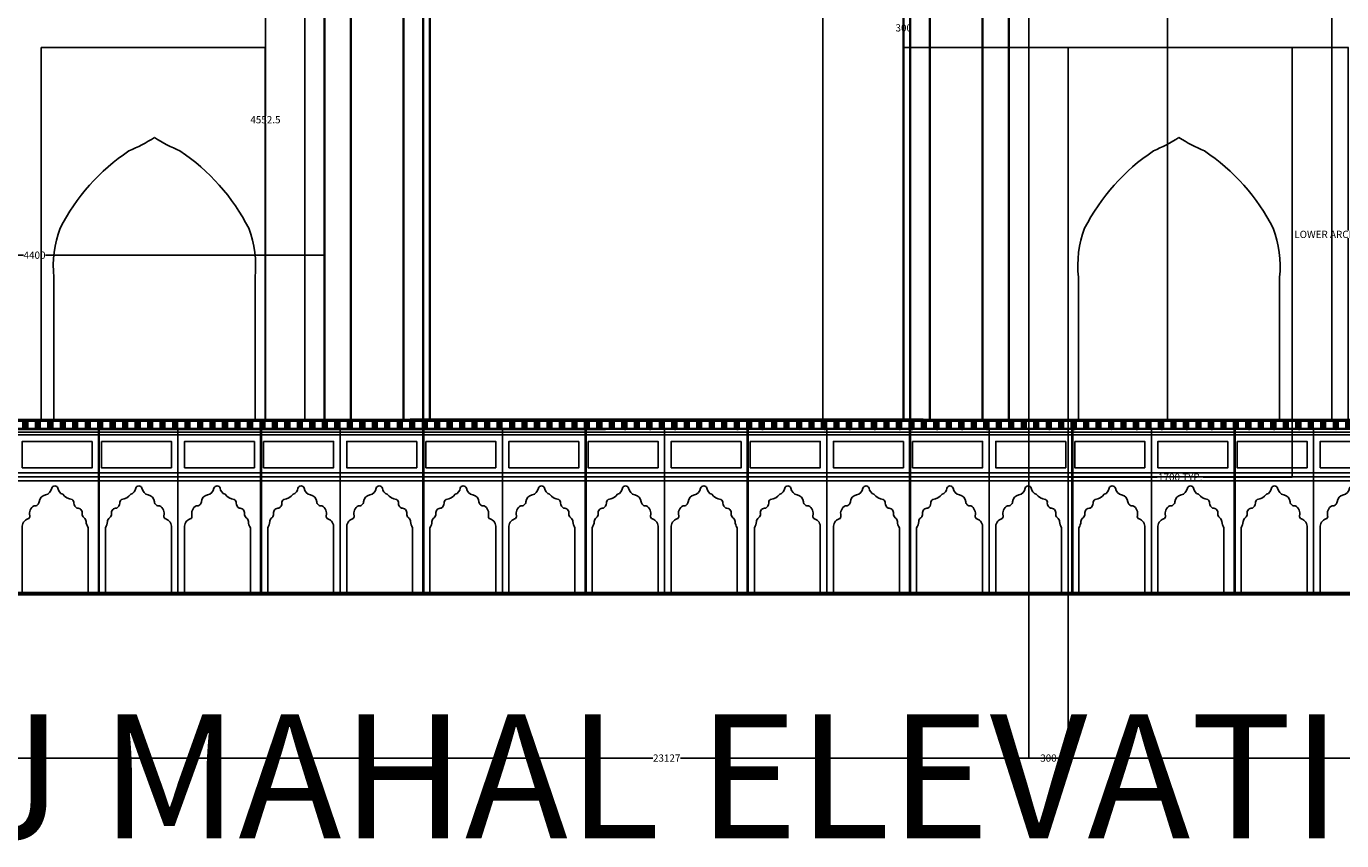
# Model space of a CAD drawing. Units: millimetres. Extents: x 8570 to 49085, y 3782 to 24863.
# Tile 4 of 15: x 17549 to 27529, y 4026 to 10208. Entities that reach past the tile are written whole.
import ezdxf

# ---------------------------------------------------------------- set-up
doc = ezdxf.new("R2010")
doc.units = ezdxf.units.MM
doc.header["$MEASUREMENT"] = 0
doc.header["$PDMODE"] = 3
for name, color, linetype, lineweight in [('A-ANNO-DIMS', 2, 'Continuous', 18), ('A-ANNO-TEXT', 7, 'Continuous', 25), ('A-ELEV-ARCH', 7, 'Continuous', 25), ('A-ELEV-GRND', 7, 'Continuous', 35), ('A-ELEV-IWAN', 7, 'Continuous', 35), ('A-ELEV-PATT', 252, 'Continuous', 13), ('A-ELEV-PIER', 7, 'Continuous', 25), ('A-ELEV-PLIN', 7, 'Continuous', 25)]:
    doc.layers.add(name, color=color, linetype=linetype, lineweight=lineweight)
doc.styles.get("Standard").update_dxf_attribs({"font": 'arial.ttf'})
doc.dimstyles.get("Standard").update_dxf_attribs({"dimtxt": 55, "dimasz": 0.18, "dimexe": 0.18, "dimexo": 0.0625, "dimgap": 0.09, "dimtad": 0, "dimtih": 1, "dimtoh": 1, "dimdec": 0, "dimzin": 0, "dimdsep": 46, "dimtxsty": 'Standard', "dimcen": 0.09, "dimadec": 0, "dimazin": 0, "dimtfac": 1, "dimtdec": 0, "dimtofl": 0, "dimtmove": 0, "dimatfit": 3, "dimfxl": 1, "dimtolj": 1, "dimtzin": 0, "dimarcsym": 0})

# ---------------------------------------------------------------- blocks, each defined once
blk = doc.blocks.new('PLINTH-PAIRED-BAY')
for p, q in [((623.5, 0), (623.5, 1246)), ((573.5, 0), (623.5, 0)), ((1173.5, 0), (1223.5, 0))]:
    blk.add_line(p, q)
for points in [[(0, 1309.5), (58.5, 1309.5), (58.5, 1253), (0, 1253)], [(94.7, 1309.5), (153.2, 1309.5), (153.2, 1253), (94.7, 1253)], [(189.5, 1309.5), (248, 1309.5), (248, 1253), (189.5, 1253)], [(284.2, 1309.5), (342.7, 1309.5), (342.7, 1253), (284.2, 1253)], [(378.9, 1309.5), (437.4, 1309.5), (437.4, 1253), (378.9, 1253)], [(473.7, 1309.5), (532.2, 1309.5), (532.2, 1253), (473.7, 1253)], [(568.4, 1309.5), (626.9, 1309.5), (626.9, 1253), (568.4, 1253)], [(663.2, 1309.5), (721.7, 1309.5), (721.7, 1253), (663.2, 1253)], [(757.9, 1309.5), (816.4, 1309.5), (816.4, 1253), (757.9, 1253)], [(852.6, 1309.5), (911.1, 1309.5), (911.1, 1253), (852.6, 1253)], [(947.4, 1309.5), (1005.9, 1309.5), (1005.9, 1253), (947.4, 1253)], [(1042.1, 1309.5), (1100.6, 1309.5), (1100.6, 1253), (1042.1, 1253)], [(1136.8, 1309.5), (1195.3, 1309.5), (1195.3, 1253), (1136.8, 1253)], [(42.5, 1156), (573.5, 1156), (573.5, 956), (42.5, 956)], [(1204.5, 1156), (673.5, 1156), (673.5, 956), (1204.5, 956)]]:
    blk.add_lwpolyline(points, close=True)
for points in [[(573.5, 500), (573.5, 0), (73.5, 0), (73.5, 500, 0.133896), (89, 547, -0.229833), (105, 576, 0.282739), (118.5, 607.5, -0.502693), (159, 648, 0.231145), (182, 687, -0.35399), (196, 714, 0.196071), (266.2, 753.9, 0.282071), (303.4, 799.6, -0.761042), (350.3, 800.8, 0.299945), (398, 749.1, -0.349607), (445.5, 697, 0.443472), (484, 666.5, -0.349941), (517, 591, 0.399043), (530.5, 568, -0.342474)], [(673.5, 500), (673.5, 0), (1173.5, 0), (1173.5, 500, -0.133896), (1158, 547, 0.229833), (1142, 576, -0.282739), (1128.5, 607.5, 0.502693), (1088, 648, -0.231145), (1065, 687, 0.35399), (1051, 714, -0.196071), (980.8, 753.9, -0.282071), (943.6, 799.6, 0.761042), (896.7, 800.8, -0.299945), (849, 749.1, 0.349607), (801.5, 697, -0.443472), (763, 666.5, 0.349941), (730, 591, -0.399043), (716.5, 568, 0.342474)]]:
    blk.add_lwpolyline(points, format="xyb", close=True)
blk = doc.blocks.new('IWAN-EDGE-PINNACLE')
for p, q in [((10, 9044.5), (210, 9044.5)), ((10, 9004.5), (210, 9004.5)), ((35, 0), (35, 9004.5)), ((185, 0), (185, 9004.5))]:
    blk.add_line(p, q)
blk.add_lwpolyline([(127.1, 9142.4, 0.216309), (108.4, 9173.9, 0.244698), (89.5, 9137.5, 0.244698)], format="xyb")
blk.add_circle((110.5, 9116), 7.02)
for centre, radius, start, end in [((-119.7, 9355.4), 336.9, 292.6494, 312.99463), ((108.1, 9141.9), 19, 193.30654, 1.38797), ((340.2, 9356.1), 337.7, 227.0303, 247.32566), ((10, 9034.5), 10, 90, 270), ((10, 9014.5), 10, 90, 270), ((210, 9034.5), 10, 270, 90), ((210, 9014.5), 10, 270, 90)]:
    blk.add_arc(centre, radius, start, end)
blk = doc.blocks.new('PAVILION-EDGE-PINNACLE')
for p, q in [((10, 8089.5), (160, 8089.5)), ((10, 0), (10, 8069.5)), ((10, 8069.5), (160, 8069.5)), ((160, 0), (160, 8069.5)), ((160, 0), (160, 6876.5)), ((10, 0), (10, 6246.5))]:
    blk.add_line(p, q)
blk.add_lwpolyline([(101.6, 8204.8, 0.216309), (82.9, 8236.3, 0.244698), (64, 8200, 0.244698)], format="xyb")
for centre, radius, start, end in [((153, 8055.1), 147, 117.52778, 166.47476), ((82.6, 8204.4), 19, 193.30654, 1.38797), ((17, 8055.1), 147, 13.52524, 62.47222), ((10, 8079.5), 10, 90, 270), ((160, 8079.5), 10, 270, 90)]:
    blk.add_arc(centre, radius, start, end)
blk = doc.blocks.new('WING-LOWER-ARCH')
for p, q in [((0, 11.5), (0, 2834.8)), ((0, 2834.8), (1700, 2834.8)), ((1700, 11.5), (1700, 2834.8)), ((76.8, 0), (76.8, 1091.8)), ((1603.6, 0), (1603.6, 1091.8))]:
    blk.add_line(p, q)
for points in [[(124.7, 1463.8, -0.128405), (646.4, 2050.4, 0.03556), (840.2, 2151.4)], [(1555.7, 1463.8, 0.128405), (1034, 2050.4, -0.03556), (840.2, 2151.4)]]:
    blk.add_lwpolyline(points, format="xyb")
for centre, start, end in [((894.2, 1175.6), 159.46554, 185.85431), ((786.2, 1175.6), 354.14569, 20.53446)]:
    blk.add_arc(centre, 821.7, start, end)
blk = doc.blocks.new('*D19')
at = {"layer": 'A-ANNO-DIMS', "color": 0, "lineweight": -2, "transparency": 16777216}
for p, q in [((24968.9, 16396.4), (23592.7, 16396.4)), ((23592.9, 16396.2), (23592.9, 11838)), ((23592.9, 7222.7), (23592.9, 11780.9)), ((24968.9, 7222.5), (23592.7, 7222.5))]:
    blk.add_line(p, q, dxfattribs=at)
at = {"layer": 'A-ANNO-DIMS', "color": 0, "transparency": 16777216}
for points in [[(23592.9, 16396.2), (23593, 16396.2), (23592.9, 16396.4)], [(23592.9, 7222.7), (23593, 7222.7), (23592.9, 7222.5)]]:
    blk.add_solid(points, dxfattribs=at)
at = {"layer": 'Defpoints', "color": 0, "transparency": 16777216}
for p in [(23592.9, 16396.4), (24969, 16396.4), (24969, 7222.5)]:
    blk.add_point(p, dxfattribs=at)
at = {"layer": 'A-ANNO-DIMS', "color": 0, "transparency": 16777216, "insert": (23592.9, 11809.4), "char_height": 55, "attachment_point": 5}
blk.add_mtext('\\A1;IWAN PINNACLE 9174 TYP.', dxfattribs=at)
blk = doc.blocks.new('*D21')
at = {"layer": 'A-ANNO-DIMS', "color": 0, "lineweight": -2, "transparency": 16777216}
for p, q in [((27443.9, 15458.8), (26208.4, 15458.8)), ((26208.5, 15458.7), (26208.5, 11369.2)), ((26208.5, 7222.7), (26208.5, 11312.1)), ((27443.9, 7222.5), (26208.4, 7222.5))]:
    blk.add_line(p, q, dxfattribs=at)
at = {"layer": 'A-ANNO-DIMS', "color": 0, "transparency": 16777216}
for points in [[(26208.5, 15458.7), (26208.6, 15458.7), (26208.5, 15458.8)], [(26208.5, 7222.7), (26208.6, 7222.7), (26208.5, 7222.5)]]:
    blk.add_solid(points, dxfattribs=at)
at = {"layer": 'Defpoints', "color": 0, "transparency": 16777216}
for p in [(26208.5, 15458.8), (27444, 15458.8), (27444, 7222.5)]:
    blk.add_point(p, dxfattribs=at)
at = {"layer": 'A-ANNO-DIMS', "color": 0, "transparency": 16777216, "insert": (26208.5, 11340.7), "char_height": 55, "attachment_point": 5}
blk.add_mtext('\\A1;PAVILION PINNACLE 8236 TYP.', dxfattribs=at)
blk = doc.blocks.new('*D29')
at = {"layer": 'A-ANNO-DIMS', "color": 0, "lineweight": -2, "transparency": 16777216}
for p, q in [((27154.1, 10045.8), (27579.4, 10045.8)), ((27579.2, 10045.6), (27579.2, 8656.9)), ((27579.2, 7211.2), (27579.2, 8599.8)), ((27154.1, 7211), (27579.4, 7211))]:
    blk.add_line(p, q, dxfattribs=at)
at = {"layer": 'A-ANNO-DIMS', "color": 0, "transparency": 16777216}
for points in [[(27579.2, 10045.6), (27579.2, 10045.6), (27579.2, 10045.8)], [(27579.2, 7211.2), (27579.2, 7211.2), (27579.2, 7211)]]:
    blk.add_solid(points, dxfattribs=at)
at = {"layer": 'Defpoints', "color": 0, "transparency": 16777216}
for p in [(27154, 10045.8), (27579.2, 10045.8), (27154, 7211)]:
    blk.add_point(p, dxfattribs=at)
at = {"layer": 'A-ANNO-DIMS', "color": 0, "transparency": 16777216, "insert": (27579.2, 8628.4), "char_height": 55, "attachment_point": 5}
blk.add_mtext('\\A1;LOWER ARCH 2835 TYP.', dxfattribs=at)
blk = doc.blocks.new('*D30')
at = {"layer": 'A-ANNO-DIMS', "color": 0, "lineweight": -2, "transparency": 16777216}
for p, q in [((25454, 7210.9), (25454, 6785.6)), ((27154, 7210.9), (27154, 6785.6)), ((25454.2, 6785.8), (26129.9, 6785.8)), ((27153.8, 6785.8), (26478.1, 6785.8))]:
    blk.add_line(p, q, dxfattribs=at)
at = {"layer": 'A-ANNO-DIMS', "color": 0, "transparency": 16777216}
for points in [[(25454.2, 6785.8), (25454.2, 6785.8), (25454, 6785.8)], [(27153.8, 6785.8), (27153.8, 6785.8), (27154, 6785.8)]]:
    blk.add_solid(points, dxfattribs=at)
at = {"layer": 'Defpoints', "color": 0, "transparency": 16777216}
for p in [(25454, 7211), (27154, 7211), (27154, 6785.8)]:
    blk.add_point(p, dxfattribs=at)
at = {"layer": 'A-ANNO-DIMS', "color": 0, "transparency": 16777216, "insert": (26304, 6785.8), "char_height": 55, "attachment_point": 5}
blk.add_mtext('\\A1;1700 TYP.', dxfattribs=at)
blk = doc.blocks.new('*D43')
at = {"layer": 'A-ANNO-DIMS', "color": 0, "lineweight": -2, "transparency": 16777216}
for p, q in [((10844, 5901.4), (10844, 4653.3)), ((33971, 5901.4), (33971, 4653.3)), ((10844.2, 4653.5), (22303.5, 4653.5)), ((33970.8, 4653.5), (22511.5, 4653.5))]:
    blk.add_line(p, q, dxfattribs=at)
at = {"layer": 'A-ANNO-DIMS', "color": 0, "transparency": 16777216}
for points in [[(10844.2, 4653.5), (10844.2, 4653.5), (10844, 4653.5)], [(33970.8, 4653.5), (33970.8, 4653.5), (33971, 4653.5)]]:
    blk.add_solid(points, dxfattribs=at)
at = {"layer": 'Defpoints', "color": 0, "transparency": 16777216}
for p in [(10844, 5901.5), (33971, 5901.5), (33971, 4653.5)]:
    blk.add_point(p, dxfattribs=at)
at = {"layer": 'A-ANNO-DIMS', "color": 0, "transparency": 16777216, "insert": (22407.5, 4653.5), "char_height": 55, "attachment_point": 5}
blk.add_mtext('\\A1;23127', dxfattribs=at)
blk = doc.blocks.new('*D44')
at = {"layer": 'A-ANNO-DIMS', "color": 0, "lineweight": -2, "transparency": 16777216}
for p, q in [((22399.7, 24863), (8684.3, 24863)), ((8684.5, 24862.8), (8684.5, 15410.4)), ((8684.5, 5901.7), (8684.5, 15354.1)), ((10843.9, 5901.5), (8684.3, 5901.5))]:
    blk.add_line(p, q, dxfattribs=at)
at = {"layer": 'A-ANNO-DIMS', "color": 0, "transparency": 16777216}
for points in [[(8684.5, 24862.8), (8684.5, 24862.8), (8684.5, 24863)], [(8684.5, 5901.7), (8684.5, 5901.7), (8684.5, 5901.5)]]:
    blk.add_solid(points, dxfattribs=at)
at = {"layer": 'Defpoints', "color": 0, "transparency": 16777216}
for p in [(8684.5, 24863), (22399.8, 24863), (10844, 5901.5)]:
    blk.add_point(p, dxfattribs=at)
at = {"layer": 'A-ANNO-DIMS', "color": 0, "transparency": 16777216, "insert": (8684.5, 15382.2), "char_height": 55, "attachment_point": 5}
blk.add_mtext('\\A1;18961', dxfattribs=at)
blk = doc.blocks.new('*D46')
at = {"layer": 'A-ANNO-DIMS', "color": 0, "lineweight": -2, "transparency": 16777216}
for p, q in [((15411, 7222.6), (15411, 8470.7)), ((15411.2, 8470.5), (17527.8, 8470.5)), ((19810.8, 8470.5), (17694.2, 8470.5)), ((19811, 7222.6), (19811, 8470.7))]:
    blk.add_line(p, q, dxfattribs=at)
at = {"layer": 'A-ANNO-DIMS', "color": 0, "transparency": 16777216}
for points in [[(15411.2, 8470.5), (15411.2, 8470.5), (15411, 8470.5)], [(19810.8, 8470.5), (19810.8, 8470.5), (19811, 8470.5)]]:
    blk.add_solid(points, dxfattribs=at)
at = {"layer": 'Defpoints', "color": 0, "transparency": 16777216}
for p in [(19811, 8470.5), (15411, 7222.5), (19811, 7222.5)]:
    blk.add_point(p, dxfattribs=at)
at = {"layer": 'A-ANNO-DIMS', "color": 0, "transparency": 16777216, "insert": (17611, 8470.5), "char_height": 55, "attachment_point": 5}
blk.add_mtext('\\A1;4400', dxfattribs=at)
blk = doc.blocks.new('*D49')
at = {"layer": 'A-ANNO-DIMS', "color": 0, "lineweight": -2, "transparency": 16777216}
for p, q in [((20610.9, 11775), (19362.8, 11775)), ((19363, 11774.8), (19363, 9526.9)), ((19363, 7222.7), (19363, 9470.6)), ((20610.9, 7222.5), (19362.8, 7222.5))]:
    blk.add_line(p, q, dxfattribs=at)
at = {"layer": 'A-ANNO-DIMS', "color": 0, "transparency": 16777216}
for points in [[(19363, 11774.8), (19363, 11774.8), (19363, 11775)], [(19363, 7222.7), (19363, 7222.7), (19363, 7222.5)]]:
    blk.add_solid(points, dxfattribs=at)
at = {"layer": 'Defpoints', "color": 0, "transparency": 16777216}
for p in [(19363, 11775), (20611, 11775), (20611, 7222.5)]:
    blk.add_point(p, dxfattribs=at)
at = {"layer": 'A-ANNO-DIMS', "color": 0, "transparency": 16777216, "insert": (19363, 9498.7), "char_height": 55, "attachment_point": 5}
blk.add_mtext('\\A1;4552.5', dxfattribs=at)
blk = doc.blocks.new('*D59')
at = {"layer": 'A-ANNO-DIMS', "color": 0, "lineweight": -2, "transparency": 16777216}
for p, q in [((32990.4, 10606.5), (8684.3, 10606.5)), ((8684.5, 10606.3), (8684.5, 8942.7)), ((8684.5, 7222.7), (8684.5, 8886.3)), ((32870.9, 7222.5), (8684.3, 7222.5))]:
    blk.add_line(p, q, dxfattribs=at)
at = {"layer": 'A-ANNO-DIMS', "color": 0, "transparency": 16777216}
for points in [[(8684.5, 10606.3), (8684.5, 10606.3), (8684.5, 10606.5)], [(8684.5, 7222.7), (8684.5, 7222.7), (8684.5, 7222.5)]]:
    blk.add_solid(points, dxfattribs=at)
at = {"layer": 'Defpoints', "color": 0, "transparency": 16777216}
for p in [(8684.5, 10606.5), (32990.5, 10606.5), (32871, 7222.5)]:
    blk.add_point(p, dxfattribs=at)
at = {"layer": 'A-ANNO-DIMS', "color": 0, "transparency": 16777216, "insert": (8684.5, 8914.5), "char_height": 55, "attachment_point": 5}
blk.add_mtext('\\A1;3384', dxfattribs=at)
blk = doc.blocks.new('*D66')
at = {"layer": 'A-ANNO-DIMS', "color": 0, "lineweight": -2, "transparency": 16777216}
for p, q in [((25453.9, 10345.8), (24205.8, 10345.8)), ((24206, 10345.6), (24206, 10223.9)), ((24206, 10045.9), (24206, 10167.6)), ((25453.9, 10045.8), (24205.8, 10045.8))]:
    blk.add_line(p, q, dxfattribs=at)
at = {"layer": 'A-ANNO-DIMS', "color": 0, "transparency": 16777216}
for points in [[(24206, 10345.6), (24206, 10345.6), (24206, 10345.8)], [(24206, 10045.9), (24206, 10045.9), (24206, 10045.8)]]:
    blk.add_solid(points, dxfattribs=at)
at = {"layer": 'Defpoints', "color": 0, "transparency": 16777216}
for p in [(24206, 10345.8), (25454, 10345.8), (25454, 10045.8)]:
    blk.add_point(p, dxfattribs=at)
at = {"layer": 'A-ANNO-DIMS', "color": 0, "transparency": 16777216, "insert": (24206, 10195.7), "char_height": 55, "attachment_point": 5}
blk.add_mtext('\\A1;300', dxfattribs=at)
blk = doc.blocks.new('*D70')
at = {"layer": 'A-ANNO-DIMS', "color": 0, "lineweight": -2, "transparency": 16777216}
for p, q in [((25154, 7222.4), (25154, 4653.3)), ((25454, 7222.4), (25454, 4653.3)), ((25154.2, 4653.5), (25243.3, 4653.5)), ((25453.8, 4653.5), (25364.7, 4653.5))]:
    blk.add_line(p, q, dxfattribs=at)
at = {"layer": 'A-ANNO-DIMS', "color": 0, "transparency": 16777216}
for points in [[(25154.2, 4653.5), (25154.2, 4653.5), (25154, 4653.5)], [(25453.8, 4653.5), (25453.8, 4653.5), (25454, 4653.5)]]:
    blk.add_solid(points, dxfattribs=at)
at = {"layer": 'Defpoints', "color": 0, "transparency": 16777216}
for p in [(25154, 7222.5), (25454, 7222.5), (25454, 4653.5)]:
    blk.add_point(p, dxfattribs=at)
at = {"layer": 'A-ANNO-DIMS', "color": 0, "transparency": 16777216, "insert": (25304, 4653.5), "char_height": 55, "attachment_point": 5}
blk.add_mtext('\\A1;300', dxfattribs=at)

msp = doc.modelspace()

# ---------------------------------------------------------------- hatches: boundary and pattern name
at = {"layer": 'A-ELEV-PATT'}
h = msp.add_hatch(dxfattribs=at)
h.set_pattern_fill('ANSI31', color=256)
h.set_pattern_definition([(45, (3693, 0), (-0.0883883476, 0.0883883476), [])])
h.paths.add_polyline_path([(16868, 7222.5), (18099, 7222.5), (18099, 7147.5), (16868, 7147.5)])
h.paths.add_polyline_path([(17180.37, 7154.5), (17238.87, 7154.5), (17238.87, 7211), (17180.37, 7211)], flags=16)
h.paths.add_polyline_path([(17144.13, 7211), (17085.63, 7211), (17085.63, 7154.5), (17144.13, 7154.5)], flags=16)
h.paths.add_polyline_path([(17275.11, 7154.5), (17333.61, 7154.5), (17333.61, 7211), (17275.11, 7211)], flags=16)
h.paths.add_polyline_path([(17049.39, 7211), (16990.89, 7211), (16990.89, 7154.5), (17049.39, 7154.5)], flags=16)
h.paths.add_polyline_path([(17369.84, 7154.5), (17428.34, 7154.5), (17428.34, 7211), (17369.84, 7211)], flags=16)
h.paths.add_polyline_path([(16954.66, 7211), (16896.16, 7211), (16896.16, 7154.5), (16954.66, 7154.5)], flags=16)
h.paths.add_polyline_path([(17464.58, 7154.5), (17523.08, 7154.5), (17523.08, 7211), (17464.58, 7211)], flags=16)
h.paths.add_polyline_path([(17559.32, 7154.5), (17617.82, 7154.5), (17617.82, 7211), (17559.32, 7211)], flags=16)
h.paths.add_polyline_path([(17654.05, 7154.5), (17712.55, 7154.5), (17712.55, 7211), (17654.05, 7211)], flags=16)
h.paths.add_polyline_path([(17748.79, 7154.5), (17807.29, 7154.5), (17807.29, 7211), (17748.79, 7211)], flags=16)
h.paths.add_polyline_path([(17843.53, 7154.5), (17902.03, 7154.5), (17902.03, 7211), (17843.53, 7211)], flags=16)
h.paths.add_polyline_path([(17938.26, 7154.5), (17996.76, 7154.5), (17996.76, 7211), (17938.26, 7211)], flags=16)
h.paths.add_polyline_path([(18033, 7154.5), (18091.5, 7154.5), (18091.5, 7211), (18033, 7211)], flags=16)
h = msp.add_hatch(dxfattribs=at)
h.set_pattern_fill('ANSI31', color=256)
h.set_pattern_definition([(45, (4924, 0), (-0.0883883476, 0.0883883476), [])])
h.paths.add_polyline_path([(18099, 7222.5), (19330, 7222.5), (19330, 7147.5), (18099, 7147.5)])
h.paths.add_polyline_path([(18411.37, 7154.5), (18469.87, 7154.5), (18469.87, 7211), (18411.37, 7211)], flags=16)
h.paths.add_polyline_path([(18375.13, 7211), (18316.63, 7211), (18316.63, 7154.5), (18375.13, 7154.5)], flags=16)
h.paths.add_polyline_path([(18506.11, 7154.5), (18564.61, 7154.5), (18564.61, 7211), (18506.11, 7211)], flags=16)
h.paths.add_polyline_path([(18280.39, 7211), (18221.89, 7211), (18221.89, 7154.5), (18280.39, 7154.5)], flags=16)
h.paths.add_polyline_path([(18600.84, 7154.5), (18659.34, 7154.5), (18659.34, 7211), (18600.84, 7211)], flags=16)
h.paths.add_polyline_path([(18185.66, 7211), (18127.16, 7211), (18127.16, 7154.5), (18185.66, 7154.5)], flags=16)
h.paths.add_polyline_path([(18695.58, 7154.5), (18754.08, 7154.5), (18754.08, 7211), (18695.58, 7211)], flags=16)
h.paths.add_polyline_path([(18790.32, 7154.5), (18848.82, 7154.5), (18848.82, 7211), (18790.32, 7211)], flags=16)
h.paths.add_polyline_path([(18885.05, 7154.5), (18943.55, 7154.5), (18943.55, 7211), (18885.05, 7211)], flags=16)
h.paths.add_polyline_path([(18979.79, 7154.5), (19038.29, 7154.5), (19038.29, 7211), (18979.79, 7211)], flags=16)
h.paths.add_polyline_path([(19074.53, 7154.5), (19133.03, 7154.5), (19133.03, 7211), (19074.53, 7211)], flags=16)
h.paths.add_polyline_path([(19169.26, 7154.5), (19227.76, 7154.5), (19227.76, 7211), (19169.26, 7211)], flags=16)
h.paths.add_polyline_path([(19264, 7154.5), (19322.5, 7154.5), (19322.5, 7211), (19264, 7211)], flags=16)
h = msp.add_hatch(dxfattribs=at)
h.set_pattern_fill('ANSI31', color=256)
h.set_pattern_definition([(45, (6155, 0), (-0.0883883476, 0.0883883476), [])])
h.paths.add_polyline_path([(19330, 7222.5), (20561, 7222.5), (20561, 7147.5), (19330, 7147.5)])
h.paths.add_polyline_path([(19642.37, 7154.5), (19700.87, 7154.5), (19700.87, 7211), (19642.37, 7211)], flags=16)
h.paths.add_polyline_path([(19606.13, 7211), (19547.63, 7211), (19547.63, 7154.5), (19606.13, 7154.5)], flags=16)
h.paths.add_polyline_path([(19737.11, 7154.5), (19795.61, 7154.5), (19795.61, 7211), (19737.11, 7211)], flags=16)
h.paths.add_polyline_path([(19511.39, 7211), (19452.89, 7211), (19452.89, 7154.5), (19511.39, 7154.5)], flags=16)
h.paths.add_polyline_path([(19831.84, 7154.5), (19890.34, 7154.5), (19890.34, 7211), (19831.84, 7211)], flags=16)
h.paths.add_polyline_path([(19416.66, 7211), (19358.16, 7211), (19358.16, 7154.5), (19416.66, 7154.5)], flags=16)
h.paths.add_polyline_path([(19926.58, 7154.5), (19985.08, 7154.5), (19985.08, 7211), (19926.58, 7211)], flags=16)
h.paths.add_polyline_path([(20021.32, 7154.5), (20079.82, 7154.5), (20079.82, 7211), (20021.32, 7211)], flags=16)
h.paths.add_polyline_path([(20116.05, 7154.5), (20174.55, 7154.5), (20174.55, 7211), (20116.05, 7211)], flags=16)
h.paths.add_polyline_path([(20210.79, 7154.5), (20269.29, 7154.5), (20269.29, 7211), (20210.79, 7211)], flags=16)
h.paths.add_polyline_path([(20305.53, 7154.5), (20364.03, 7154.5), (20364.03, 7211), (20305.53, 7211)], flags=16)
h.paths.add_polyline_path([(20400.26, 7154.5), (20458.76, 7154.5), (20458.76, 7211), (20400.26, 7211)], flags=16)
h.paths.add_polyline_path([(20495, 7154.5), (20553.5, 7154.5), (20553.5, 7211), (20495, 7211)], flags=16)
h = msp.add_hatch(dxfattribs=at)
h.set_pattern_fill('ANSI31', color=256)
h.set_pattern_definition([(45, (7386, 0), (-0.0883883476, 0.0883883476), [])])
h.paths.add_polyline_path([(20561, 7222.5), (21792, 7222.5), (21792, 7147.5), (20561, 7147.5)])
h.paths.add_polyline_path([(20873.37, 7154.5), (20931.87, 7154.5), (20931.87, 7211), (20873.37, 7211)], flags=16)
h.paths.add_polyline_path([(20837.13, 7211), (20778.63, 7211), (20778.63, 7154.5), (20837.13, 7154.5)], flags=16)
h.paths.add_polyline_path([(20968.11, 7154.5), (21026.61, 7154.5), (21026.61, 7211), (20968.11, 7211)], flags=16)
h.paths.add_polyline_path([(20742.39, 7211), (20683.89, 7211), (20683.89, 7154.5), (20742.39, 7154.5)], flags=16)
h.paths.add_polyline_path([(21062.84, 7154.5), (21121.34, 7154.5), (21121.34, 7211), (21062.84, 7211)], flags=16)
h.paths.add_polyline_path([(20647.66, 7211), (20589.16, 7211), (20589.16, 7154.5), (20647.66, 7154.5)], flags=16)
h.paths.add_polyline_path([(21157.58, 7154.5), (21216.08, 7154.5), (21216.08, 7211), (21157.58, 7211)], flags=16)
h.paths.add_polyline_path([(21252.32, 7154.5), (21310.82, 7154.5), (21310.82, 7211), (21252.32, 7211)], flags=16)
h.paths.add_polyline_path([(21347.05, 7154.5), (21405.55, 7154.5), (21405.55, 7211), (21347.05, 7211)], flags=16)
h.paths.add_polyline_path([(21441.79, 7154.5), (21500.29, 7154.5), (21500.29, 7211), (21441.79, 7211)], flags=16)
h.paths.add_polyline_path([(21536.53, 7154.5), (21595.03, 7154.5), (21595.03, 7211), (21536.53, 7211)], flags=16)
h.paths.add_polyline_path([(21631.26, 7154.5), (21689.76, 7154.5), (21689.76, 7211), (21631.26, 7211)], flags=16)
h.paths.add_polyline_path([(21726, 7154.5), (21784.5, 7154.5), (21784.5, 7211), (21726, 7211)], flags=16)
h = msp.add_hatch(dxfattribs=at)
h.set_pattern_fill('ANSI31', color=256)
h.set_pattern_definition([(45, (8617, 0), (-0.0883883476, 0.0883883476), [])])
h.paths.add_polyline_path([(21792, 7222.5), (23023, 7222.5), (23023, 7147.5), (21792, 7147.5)])
h.paths.add_polyline_path([(22104.37, 7154.5), (22162.87, 7154.5), (22162.87, 7211), (22104.37, 7211)], flags=16)
h.paths.add_polyline_path([(22068.13, 7211), (22009.63, 7211), (22009.63, 7154.5), (22068.13, 7154.5)], flags=16)
h.paths.add_polyline_path([(22199.11, 7154.5), (22257.61, 7154.5), (22257.61, 7211), (22199.11, 7211)], flags=16)
h.paths.add_polyline_path([(21973.39, 7211), (21914.89, 7211), (21914.89, 7154.5), (21973.39, 7154.5)], flags=16)
h.paths.add_polyline_path([(22293.84, 7154.5), (22352.34, 7154.5), (22352.34, 7211), (22293.84, 7211)], flags=16)
h.paths.add_polyline_path([(21878.66, 7211), (21820.16, 7211), (21820.16, 7154.5), (21878.66, 7154.5)], flags=16)
h.paths.add_polyline_path([(22388.58, 7154.5), (22447.08, 7154.5), (22447.08, 7211), (22388.58, 7211)], flags=16)
h.paths.add_polyline_path([(22483.32, 7154.5), (22541.82, 7154.5), (22541.82, 7211), (22483.32, 7211)], flags=16)
h.paths.add_polyline_path([(22578.05, 7154.5), (22636.55, 7154.5), (22636.55, 7211), (22578.05, 7211)], flags=16)
h.paths.add_polyline_path([(22672.79, 7154.5), (22731.29, 7154.5), (22731.29, 7211), (22672.79, 7211)], flags=16)
h.paths.add_polyline_path([(22767.53, 7154.5), (22826.03, 7154.5), (22826.03, 7211), (22767.53, 7211)], flags=16)
h.paths.add_polyline_path([(22862.26, 7154.5), (22920.76, 7154.5), (22920.76, 7211), (22862.26, 7211)], flags=16)
h.paths.add_polyline_path([(22957, 7154.5), (23015.5, 7154.5), (23015.5, 7211), (22957, 7211)], flags=16)
h = msp.add_hatch(dxfattribs=at)
h.set_pattern_fill('ANSI31', color=256)
h.set_pattern_definition([(45, (9848, 0), (-0.0883883476, 0.0883883476), [])])
h.paths.add_polyline_path([(23023, 7222.5), (24254, 7222.5), (24254, 7147.5), (23023, 7147.5)])
h.paths.add_polyline_path([(23335.37, 7154.5), (23393.87, 7154.5), (23393.87, 7211), (23335.37, 7211)], flags=16)
h.paths.add_polyline_path([(23299.13, 7211), (23240.63, 7211), (23240.63, 7154.5), (23299.13, 7154.5)], flags=16)
h.paths.add_polyline_path([(23430.11, 7154.5), (23488.61, 7154.5), (23488.61, 7211), (23430.11, 7211)], flags=16)
h.paths.add_polyline_path([(23204.39, 7211), (23145.89, 7211), (23145.89, 7154.5), (23204.39, 7154.5)], flags=16)
h.paths.add_polyline_path([(23524.84, 7154.5), (23583.34, 7154.5), (23583.34, 7211), (23524.84, 7211)], flags=16)
h.paths.add_polyline_path([(23109.66, 7211), (23051.16, 7211), (23051.16, 7154.5), (23109.66, 7154.5)], flags=16)
h.paths.add_polyline_path([(23619.58, 7154.5), (23678.08, 7154.5), (23678.08, 7211), (23619.58, 7211)], flags=16)
h.paths.add_polyline_path([(23714.32, 7154.5), (23772.82, 7154.5), (23772.82, 7211), (23714.32, 7211)], flags=16)
h.paths.add_polyline_path([(23809.05, 7154.5), (23867.55, 7154.5), (23867.55, 7211), (23809.05, 7211)], flags=16)
h.paths.add_polyline_path([(23903.79, 7154.5), (23962.29, 7154.5), (23962.29, 7211), (23903.79, 7211)], flags=16)
h.paths.add_polyline_path([(23998.53, 7154.5), (24057.03, 7154.5), (24057.03, 7211), (23998.53, 7211)], flags=16)
h.paths.add_polyline_path([(24093.26, 7154.5), (24151.76, 7154.5), (24151.76, 7211), (24093.26, 7211)], flags=16)
h.paths.add_polyline_path([(24188, 7154.5), (24246.5, 7154.5), (24246.5, 7211), (24188, 7211)], flags=16)
h = msp.add_hatch(dxfattribs=at)
h.set_pattern_fill('ANSI31', color=256)
h.set_pattern_definition([(45, (11079, 0), (-0.0883883476, 0.0883883476), [])])
h.paths.add_polyline_path([(24254, 7222.5), (25485, 7222.5), (25485, 7147.5), (24254, 7147.5)])
h.paths.add_polyline_path([(24566.37, 7154.5), (24624.87, 7154.5), (24624.87, 7211), (24566.37, 7211)], flags=16)
h.paths.add_polyline_path([(24530.13, 7211), (24471.63, 7211), (24471.63, 7154.5), (24530.13, 7154.5)], flags=16)
h.paths.add_polyline_path([(24661.11, 7154.5), (24719.61, 7154.5), (24719.61, 7211), (24661.11, 7211)], flags=16)
h.paths.add_polyline_path([(24435.39, 7211), (24376.89, 7211), (24376.89, 7154.5), (24435.39, 7154.5)], flags=16)
h.paths.add_polyline_path([(24755.84, 7154.5), (24814.34, 7154.5), (24814.34, 7211), (24755.84, 7211)], flags=16)
h.paths.add_polyline_path([(24340.66, 7211), (24282.16, 7211), (24282.16, 7154.5), (24340.66, 7154.5)], flags=16)
h.paths.add_polyline_path([(24850.58, 7154.5), (24909.08, 7154.5), (24909.08, 7211), (24850.58, 7211)], flags=16)
h.paths.add_polyline_path([(24945.32, 7154.5), (25003.82, 7154.5), (25003.82, 7211), (24945.32, 7211)], flags=16)
h.paths.add_polyline_path([(25040.05, 7154.5), (25098.55, 7154.5), (25098.55, 7211), (25040.05, 7211)], flags=16)
h.paths.add_polyline_path([(25134.79, 7154.5), (25193.29, 7154.5), (25193.29, 7211), (25134.79, 7211)], flags=16)
h.paths.add_polyline_path([(25229.53, 7154.5), (25288.03, 7154.5), (25288.03, 7211), (25229.53, 7211)], flags=16)
h.paths.add_polyline_path([(25324.26, 7154.5), (25382.76, 7154.5), (25382.76, 7211), (25324.26, 7211)], flags=16)
h.paths.add_polyline_path([(25419, 7154.5), (25477.5, 7154.5), (25477.5, 7211), (25419, 7211)], flags=16)
h = msp.add_hatch(dxfattribs=at)
h.set_pattern_fill('ANSI31', color=256)
h.set_pattern_definition([(45, (12310, 0), (-0.0883883476, 0.0883883476), [])])
h.paths.add_polyline_path([(25485, 7222.5), (26716, 7222.5), (26716, 7147.5), (25485, 7147.5)])
h.paths.add_polyline_path([(25797.37, 7154.5), (25855.87, 7154.5), (25855.87, 7211), (25797.37, 7211)], flags=16)
h.paths.add_polyline_path([(25761.13, 7211), (25702.63, 7211), (25702.63, 7154.5), (25761.13, 7154.5)], flags=16)
h.paths.add_polyline_path([(25892.11, 7154.5), (25950.61, 7154.5), (25950.61, 7211), (25892.11, 7211)], flags=16)
h.paths.add_polyline_path([(25666.39, 7211), (25607.89, 7211), (25607.89, 7154.5), (25666.39, 7154.5)], flags=16)
h.paths.add_polyline_path([(25986.84, 7154.5), (26045.34, 7154.5), (26045.34, 7211), (25986.84, 7211)], flags=16)
h.paths.add_polyline_path([(25571.66, 7211), (25513.16, 7211), (25513.16, 7154.5), (25571.66, 7154.5)], flags=16)
h.paths.add_polyline_path([(26081.58, 7154.5), (26140.08, 7154.5), (26140.08, 7211), (26081.58, 7211)], flags=16)
h.paths.add_polyline_path([(26176.32, 7154.5), (26234.82, 7154.5), (26234.82, 7211), (26176.32, 7211)], flags=16)
h.paths.add_polyline_path([(26271.05, 7154.5), (26329.55, 7154.5), (26329.55, 7211), (26271.05, 7211)], flags=16)
h.paths.add_polyline_path([(26365.79, 7154.5), (26424.29, 7154.5), (26424.29, 7211), (26365.79, 7211)], flags=16)
h.paths.add_polyline_path([(26460.53, 7154.5), (26519.03, 7154.5), (26519.03, 7211), (26460.53, 7211)], flags=16)
h.paths.add_polyline_path([(26555.26, 7154.5), (26613.76, 7154.5), (26613.76, 7211), (26555.26, 7211)], flags=16)
h.paths.add_polyline_path([(26650, 7154.5), (26708.5, 7154.5), (26708.5, 7211), (26650, 7211)], flags=16)
h = msp.add_hatch(dxfattribs=at)
h.set_pattern_fill('ANSI31', color=256)
h.set_pattern_definition([(45, (13541, 0), (-0.0883883476, 0.0883883476), [])])
h.paths.add_polyline_path([(26716, 7222.5), (27947, 7222.5), (27947, 7147.5), (26716, 7147.5)])
h.paths.add_polyline_path([(27028.37, 7154.5), (27086.87, 7154.5), (27086.87, 7211), (27028.37, 7211)], flags=16)
h.paths.add_polyline_path([(26992.13, 7211), (26933.63, 7211), (26933.63, 7154.5), (26992.13, 7154.5)], flags=16)
h.paths.add_polyline_path([(27123.11, 7154.5), (27181.61, 7154.5), (27181.61, 7211), (27123.11, 7211)], flags=16)
h.paths.add_polyline_path([(26897.39, 7211), (26838.89, 7211), (26838.89, 7154.5), (26897.39, 7154.5)], flags=16)
h.paths.add_polyline_path([(27217.84, 7154.5), (27276.34, 7154.5), (27276.34, 7211), (27217.84, 7211)], flags=16)
h.paths.add_polyline_path([(26802.66, 7211), (26744.16, 7211), (26744.16, 7154.5), (26802.66, 7154.5)], flags=16)
h.paths.add_polyline_path([(27312.58, 7154.5), (27371.08, 7154.5), (27371.08, 7211), (27312.58, 7211)], flags=16)
h.paths.add_polyline_path([(27407.32, 7154.5), (27465.82, 7154.5), (27465.82, 7211), (27407.32, 7211)], flags=16)
h.paths.add_polyline_path([(27502.05, 7154.5), (27560.55, 7154.5), (27560.55, 7211), (27502.05, 7211)], flags=16)
h.paths.add_polyline_path([(27596.79, 7154.5), (27655.29, 7154.5), (27655.29, 7211), (27596.79, 7211)], flags=16)
h.paths.add_polyline_path([(27691.53, 7154.5), (27750.03, 7154.5), (27750.03, 7211), (27691.53, 7211)], flags=16)
h.paths.add_polyline_path([(27786.26, 7154.5), (27844.76, 7154.5), (27844.76, 7211), (27786.26, 7211)], flags=16)
h.paths.add_polyline_path([(27881, 7154.5), (27939.5, 7154.5), (27939.5, 7211), (27881, 7211)], flags=16)

# ---------------------------------------------------------------- linework, layer by layer
at = {"layer": 'A-ELEV-ARCH'}
msp.add_line((25530.77, 7211), (27057.62, 7211), dxfattribs=at)
at = {"layer": 'A-ELEV-GRND', "const_width": 30}
msp.add_lwpolyline([(9932.5, 5901.52), (34807, 5902)], dxfattribs=at)
at = {"layer": 'A-ELEV-IWAN'}
msp.add_line((20461, 7222.5), (24354, 7222.5), dxfattribs=at)
for points in [[(19811, 7222.5), (19811, 14600), (25004, 14600), (25004, 7222.5)], [(20011, 7222.5), (20011, 14400), (24804, 14400), (24804, 7222.5)], [(20411, 7222.5), (20411, 14000), (24404, 14000), (24404, 7222.5)], [(20561, 7222.5), (20561, 13850)], [(20561, 7222.5), (20561, 13850), (24254, 13850), (24254, 7222.5)], [(24254, 7222.5), (24254, 13850)], [(20611, 7222.5), (20611, 11825)], [(24204, 7222.5), (24204, 11775), (20611, 11775)]]:
    msp.add_lwpolyline(points, dxfattribs=at)
at = {"layer": 'A-ELEV-PLIN'}
for p, q in [((18099, 5901.5), (18099, 7222.5)), ((19330, 5901.5), (19330, 7222.5)), ((20561, 5901.5), (20561, 7222.5)), ((21792, 5901.5), (21792, 7222.5)), ((23023, 5901.5), (23023, 7222.5)), ((25485, 5901.5), (25485, 7222.5))]:
    msp.add_line(p, q, dxfattribs=at)
for points in [[(11944, 7222.5), (21944, 7222.5)], [(11944, 7147.5), (21944, 7147.5)], [(11944, 7127.5), (32871, 7127.5)], [(11944, 7107.5), (32871, 7107.5)], [(11944, 6817.5), (32871, 6817.5)], [(11944, 6787.5), (32871, 6787.5)], [(11944, 6757.5), (32871, 6757.5)]]:
    msp.add_lwpolyline(points, dxfattribs=at)
at = {"layer": 'A-ELEV-PLIN', "const_width": 20}
for points in [[(18099, 5901.5), (18099, 7222.5)], [(19330, 5901.5), (19330, 7222.5)], [(19330, 5901.5), (19330, 7222.5)], [(20561, 5901.5), (20561, 7222.5)], [(21792, 5901.5), (21792, 7222.5)], [(23023, 5901.5), (23023, 7222.5)], [(24254, 5901.5), (24254, 7222.5)], [(25485, 5901.5), (25485, 7222.5)], [(26716, 5901.5), (26716, 7222.5)]]:
    msp.add_lwpolyline(points, dxfattribs=at)

# ---------------------------------------------------------------- block references
at = {"layer": 'A-ELEV-ARCH', "extrusion": (0, 0, -1), "zscale": -1}
msp.add_blockref('WING-LOWER-ARCH', (-19361, 7211), dxfattribs=at)
at = {"layer": 'A-ELEV-ARCH'}
msp.add_blockref('WING-LOWER-ARCH', (25454, 7211), dxfattribs=at)
at = {"layer": 'A-ELEV-PIER', "extrusion": (0, 0, -1), "zscale": -1}
msp.add_blockref('IWAN-EDGE-PINNACLE', (-19846, 7222.5), dxfattribs=at)
at = {"layer": 'A-ELEV-PIER'}
for name, p in [('IWAN-EDGE-PINNACLE', (24969, 7222.5)), ('PAVILION-EDGE-PINNACLE', (27444, 7222.5))]:
    msp.add_blockref(name, p, dxfattribs=at)
at = {"layer": 'A-ELEV-PLIN', "extrusion": (0, 0, -1), "zscale": -1}
for p in [(-18091.5, 5901.5), (-19322.5, 5901.5), (-20553.5, 5901.5), (-21784.5, 5901.5), (-23015.5, 5901.5), (-24246.5, 5901.5), (-25477.5, 5901.5), (-26708.5, 5901.5), (-27939.5, 5901.5)]:
    msp.add_blockref('PLINTH-PAIRED-BAY', p, dxfattribs=at)

# ---------------------------------------------------------------- texts
at = {"layer": 'A-ANNO-TEXT'}
msp.add_text('TAJ MAHAL ELEVATION', height=943, dxfattribs=at).set_placement((15583.5, 4043))

# ---------------------------------------------------------------- dimensions: what is measured, and where the dimension line sits
at = {"layer": 'A-ANNO-DIMS'}
for base, p1, p2, angle, override, picture, middle in [((8684.5, 24862.95), (10844, 5901.5), (22399.75, 24862.95), 90, {"dimdec": 0, "dimlfac": 1, "dimrnd": 0, "dimzin": 0, "dimdsep": 46, "dimlunit": 2}, '*D44', (8684.5, 15382.23)), ((19363, 11775), (20611, 7222.5), (20611, 11775), 90, {"dimdec": 1, "dimlfac": 1, "dimrnd": 0, "dimzin": 0, "dimdsep": 46, "dimlunit": 2}, '*D49', (19363, 9498.75)), ((8684.5, 10606.5), (32871, 7222.5), (32990.5, 10606.5), 90, {"dimdec": 0, "dimlfac": 1, "dimrnd": 0, "dimzin": 0, "dimdsep": 46, "dimlunit": 2}, '*D59', (8684.5, 8914.5)), ((24206, 10345.75), (25454, 10045.75), (25454, 10345.75), 90, {"dimdec": 0, "dimlfac": 1, "dimrnd": 0, "dimzin": 0, "dimdsep": 46, "dimlunit": 2}, '*D66', (24206, 10195.75)), ((19811, 8470.5), (15411, 7222.5), (19811, 7222.5), 0, {"dimdec": 0, "dimlfac": 1, "dimrnd": 0, "dimzin": 0, "dimdsep": 46, "dimlunit": 2}, '*D46', (17611, 8470.5))]:
    dim = msp.add_linear_dim(base=base, p1=p1, p2=p2, angle=angle, dimstyle='Standard', override=override, dxfattribs=at)
    dim.commit()
    dim.dimension.update_dxf_attribs({"geometry": picture, "text_midpoint": middle})
for base, p1, p2, text, picture, middle in [((23592.92, 16396.36), (24969, 7222.5), (24969, 16396.36), 'IWAN PINNACLE <> TYP.', '*D19', (23592.92, 11809.43)), ((26208.55, 15458.84), (27444, 7222.5), (27444, 15458.84), 'PAVILION PINNACLE <> TYP.', '*D21', (26208.55, 11340.67)), ((27579.21, 10045.75), (27154, 7211), (27154, 10045.75), 'LOWER ARCH <> TYP.', '*D29', (27579.21, 8628.37))]:
    dim = msp.add_linear_dim(base=base, p1=p1, p2=p2, angle=90, text=text, dimstyle='Standard', override={"dimdec": 0, "dimlfac": 1, "dimrnd": 0, "dimzin": 0, "dimdsep": 46, "dimlunit": 2}, dxfattribs=at)
    dim.commit()
    dim.dimension.update_dxf_attribs({"geometry": picture, "text_midpoint": middle})
for base, p1, p2, picture, middle in [((25454, 4653.5), (25154, 7222.5), (25454, 7222.5), '*D70', (25304, 4653.5)), ((33971, 4653.5), (10844, 5901.5), (33971, 5901.5), '*D43', (22407.5, 4653.5))]:
    dim = msp.add_linear_dim(base=base, p1=p1, p2=p2, dimstyle='Standard', override={"dimdec": 0, "dimlfac": 1, "dimrnd": 0, "dimzin": 0, "dimdsep": 46, "dimlunit": 2}, dxfattribs=at)
    dim.commit()
    dim.dimension.update_dxf_attribs({"geometry": picture, "text_midpoint": middle})
dim = msp.add_linear_dim(base=(27154, 6785.79), p1=(25454, 7211), p2=(27154, 7211), text='<> TYP.', dimstyle='Standard', override={"dimdec": 0, "dimlfac": 1, "dimrnd": 0, "dimzin": 0, "dimdsep": 46, "dimlunit": 2}, dxfattribs=at)
dim.commit()
dim.dimension.update_dxf_attribs({"geometry": '*D30', "text_midpoint": (26304, 6785.79)})

doc.saveas('drawing.dxf')
